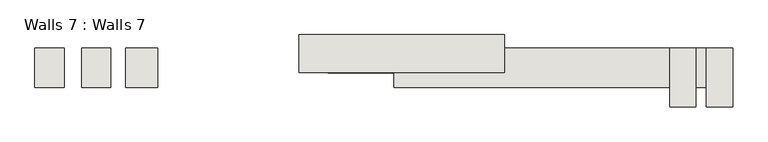
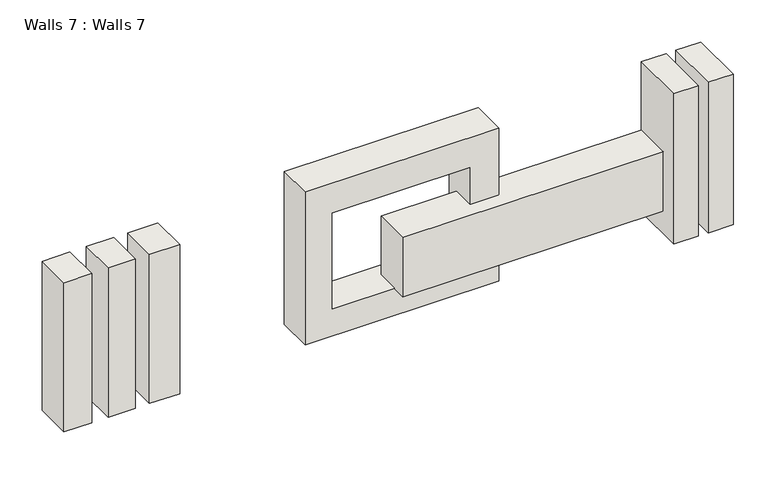
"""IFC4 building model written with IfcOpenShell, lengths in millimetres: wall geometry, Walls 7 : Walls 7."""

from ifc_helpers import new_model, si_unit, frame, origin, origin_with_axes, place, context, project, spatial, polyline, outline, extrude, source, transform, mapped, element, save


def walls_7_walls_7_e89f636e(model_context):
    return source(origin(), model_context, "Body", "SweptSolid", [
        extrude(outline(polyline([(-737.2932708, -3374.4262332), (-940.4932708, -3374.4262332), (-940.4932708, -2919.855266), (-737.2932708, -2919.855266), (-737.2932708, -3374.4262332)])), origin_with_axes(), (0.0, 0.0, 1.0), 1295.4),
        extrude(outline(polyline([(-1020.3869336, -3374.4262332), (-1219.8932708, -3374.4262332), (-1219.8932708, -2919.855266), (-1020.3869336, -2919.855266), (-1020.3869336, -3374.4262332)])), origin_with_axes(), (0.0, 0.0, 1.0), 1295.4),
        extrude(outline(polyline([(-813.4932708, -3224.655266), (-3337.3592205, -3224.655266), (-3337.3592205, -2919.855266), (-813.4932708, -2919.855266), (-813.4932708, -3224.655266)])), frame((0.0, 0.0, 196.3381352), z_axis=(0.0, 0.0, 1.0), x_axis=(1.0, 0.0, 0.0)), (0.0, 0.0, 1.0), 511.4216375),
        extrude(outline(polyline([(-5868.0932708, -3224.655266), (-6093.7940307, -3224.655266), (-6093.7940307, -2919.855266), (-5868.0932708, -2919.855266), (-5868.0932708, -3224.655266)])), origin_with_axes(), (0.0, 0.0, 1.0), 1283.88165),
        extrude(outline(polyline([(-5510.9930477, -3224.655266), (-5733.508171, -3224.655266), (-5733.508171, -2919.855266), (-5510.9930477, -2919.855266), (-5510.9930477, -3224.655266)])), origin_with_axes(), (0.0, 0.0, 1.0), 1283.88165),
        extrude(outline(polyline([(-5151.8203628, -3224.655266), (-5396.5869984, -3224.655266), (-5396.5869984, -2919.855266), (-5151.8203628, -2919.855266), (-5151.8203628, -3224.655266)])), origin_with_axes(), (0.0, 0.0, 1.0), 1283.88165),
        extrude(outline(polyline([(1283.88165, -2489.8932708), (1283.88165, -4064.6932708), (-30.56835, -4064.6932708), (-30.56835, -2489.8932708), (1283.88165, -2489.8932708)]), holes=[polyline([(1025.2624899, -2725.2396237), (203.2, -2725.2396237), (203.2, -3844.8481257), (1025.2624899, -3844.8481257), (1025.2624899, -2725.2396237)])]), frame((0.0, -3110.3864146, 0.0), z_axis=(0.0, 1.0, 0.0), x_axis=(0.0, 0.0, 1.0)), (0.0, 0.0, 1.0), 292.1311486),
    ])


if __name__ == "__main__":
    model = new_model("IFC4")
    model_context = context("Model", 3, world=origin())
    ifc_project = project(units=[si_unit("LENGTHUNIT", "METRE", prefix="MILLI")], contexts=[model_context])
    site = spatial("IfcSite", under=ifc_project)
    building = spatial("IfcBuilding", under=site)
    placement = place(None, origin())
    walls_7_walls_7_shape = walls_7_walls_7_e89f636e(model_context)
    element("IfcWall", 1, ObjectType="Walls 7 : Walls 7", at=placement, inside=building, context=model_context, shape_type="MappedRepresentation", body=[
        mapped(walls_7_walls_7_shape, transform((0.0, 0.0, 0.0), x_axis=(1.0, 0.0, 0.0), y_axis=(0.0, 1.0, 0.0), z_axis=(0.0, 0.0, 1.0))),
    ])
    save(model, "model.ifc")

# Revit data of these elements
# Element 1 (IfcWall, "Walls 7 : Walls 7")
#   Materials on its faces: "Default Wall"
# Materials
#   "Default Wall": colour RGB 128 128 128, transparency 0
